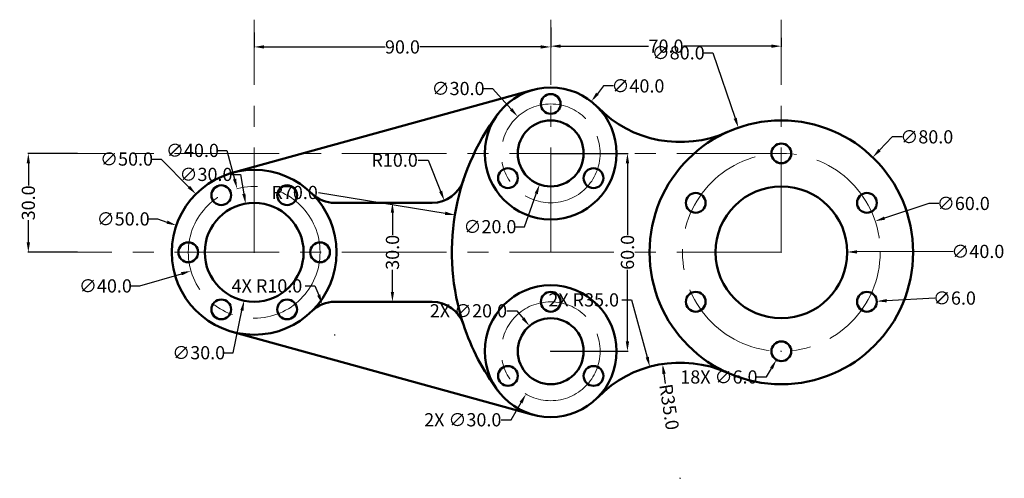
# Model space of a CAD drawing. Units: inches. Extents: x 1449 to 1748, y 643 to 782.
import ezdxf

# ---------------------------------------------------------------- set-up
doc = ezdxf.new("R2010")
doc.units = ezdxf.units.IN
doc.header["$MEASUREMENT"] = 0
doc.linetypes.add('CENTER', pattern=[50.8, 31.75, -6.35, 6.35, -6.35])
doc.layers.add('M-CNTR', color=32, linetype='CENTER', lineweight=18, true_color=0xcd6928)
doc.layers.add('M-DIMS', color=2, linetype='Continuous', lineweight=25)
doc.layers.add('M-OUTL', color=7, linetype='Continuous', lineweight=50)
doc.styles.get("Standard").update_dxf_attribs({"font": 'arial.ttf'})
doc.dimstyles.get("Standard").update_dxf_attribs({"dimtxt": 4, "dimasz": 3, "dimexe": 0.18, "dimexo": 0.0625, "dimgap": 0.09, "dimtad": 0, "dimtoh": 1, "dimdec": 1, "dimzin": 0, "dimdsep": 46, "dimtxsty": 'Standard', "dimcen": 0.09, "dimadec": 0, "dimazin": 0, "dimtfac": 1, "dimtdec": 1, "dimtofl": 0, "dimtmove": 0, "dimatfit": 3, "dimfxl": 1, "dimtolj": 1, "dimtzin": 0, "dimarcsym": 0})

# ---------------------------------------------------------------- blocks, each defined once
blk = doc.blocks.new('*D1')
at = {"layer": 'Defpoints', "color": 0, "transparency": 16777216}
for p in [(1519.9, 778.16), (1609.9, 779.72), (1609.9, 773.74)]:
    blk.add_point(p, dxfattribs=at)
at = {"layer": 'M-DIMS', "color": 0, "lineweight": -2, "transparency": 16777216}
for p, q in [((1519.9, 778.1), (1519.9, 773.56)), ((1609.9, 779.66), (1609.9, 773.56)), ((1522.9, 773.74), (1559.62, 773.74)), ((1606.9, 773.74), (1570.17, 773.74))]:
    blk.add_line(p, q, dxfattribs=at)
at = {"layer": 'M-DIMS', "color": 0, "transparency": 16777216}
for points in [[(1522.9, 774.24), (1522.9, 773.24), (1519.9, 773.74)], [(1606.9, 774.24), (1606.9, 773.24), (1609.9, 773.74)]]:
    blk.add_solid(points, dxfattribs=at)
at = {"layer": 'M-DIMS', "color": 0, "transparency": 16777216, "insert": (1564.9, 773.74), "char_height": 4, "attachment_point": 5}
blk.add_mtext('\\A1;90.0', dxfattribs=at)
blk = doc.blocks.new('*D2')
at = {"layer": 'Defpoints', "color": 0, "transparency": 16777216}
for p in [(1609.9, 776.61), (1679.9, 776.61), (1679.9, 773.98)]:
    blk.add_point(p, dxfattribs=at)
at = {"layer": 'M-DIMS', "color": 0, "lineweight": -2, "transparency": 16777216}
for p, q in [((1609.9, 776.55), (1609.9, 773.8)), ((1679.9, 776.55), (1679.9, 773.8)), ((1612.9, 773.98), (1639.63, 773.98)), ((1676.9, 773.98), (1650.16, 773.98))]:
    blk.add_line(p, q, dxfattribs=at)
at = {"layer": 'M-DIMS', "color": 0, "transparency": 16777216}
for points in [[(1612.9, 774.48), (1612.9, 773.48), (1609.9, 773.98)], [(1676.9, 774.48), (1676.9, 773.48), (1679.9, 773.98)]]:
    blk.add_solid(points, dxfattribs=at)
at = {"layer": 'M-DIMS', "color": 0, "transparency": 16777216, "insert": (1644.9, 773.98), "char_height": 4, "attachment_point": 5}
blk.add_mtext('\\A1;70.0', dxfattribs=at)
blk = doc.blocks.new('*D3')
at = {"layer": 'Defpoints', "color": 0, "transparency": 16777216}
for p in [(1609.9, 741.45), (1609.9, 681.45), (1633.19, 681.45)]:
    blk.add_point(p, dxfattribs=at)
at = {"layer": 'M-DIMS', "color": 0, "lineweight": -2, "transparency": 16777216}
for p, q in [((1609.96, 741.45), (1633.37, 741.45)), ((1633.19, 738.45), (1633.19, 716.74)), ((1633.19, 684.45), (1633.19, 706.16)), ((1609.96, 681.45), (1633.37, 681.45))]:
    blk.add_line(p, q, dxfattribs=at)
at = {"layer": 'M-DIMS', "color": 0, "transparency": 16777216}
for points in [[(1632.69, 738.45), (1633.69, 738.45), (1633.19, 741.45)], [(1632.69, 684.45), (1633.69, 684.45), (1633.19, 681.45)]]:
    blk.add_solid(points, dxfattribs=at)
at = {"layer": 'M-DIMS', "color": 0, "transparency": 16777216, "insert": (1633.19, 711.45), "char_height": 4, "attachment_point": 5, "rotation": 90}
blk.add_mtext('\\A1;60.0', dxfattribs=at)
blk = doc.blocks.new('*D4')
at = {"layer": 'Defpoints', "color": 0, "transparency": 16777216}
for p in [(1707.63, 740.27), (1652.16, 682.62)]:
    blk.add_point(p, dxfattribs=at)
at = {"layer": 'M-DIMS', "color": 0, "lineweight": -2, "transparency": 16777216}
for p, q in [((1713.59, 746.47), (1709.71, 742.44)), ((1716.59, 746.47), (1713.59, 746.47)), ((1679.81, 711.45), (1679.99, 711.45)), ((1679.9, 711.36), (1679.9, 711.54))]:
    blk.add_line(p, q, dxfattribs=at)
at = {"layer": 'M-DIMS', "color": 0, "transparency": 16777216}
blk.add_solid([(1709.35, 742.78), (1710.07, 742.09), (1707.63, 740.27)], dxfattribs=at)
at = {"layer": 'M-DIMS', "color": 0, "transparency": 16777216, "insert": (1724.05, 746.47), "char_height": 4, "attachment_point": 5}
blk.add_mtext('\\A1;∅80.0', dxfattribs=at)
blk = doc.blocks.new('*D5')
at = {"layer": 'Defpoints', "color": 0, "transparency": 16777216}
for p in [(1708.37, 720.88), (1651.42, 702.02)]:
    blk.add_point(p, dxfattribs=at)
at = {"layer": 'M-DIMS', "color": 0, "lineweight": -2, "transparency": 16777216}
for p, q in [((1724.69, 726.28), (1711.22, 721.82)), ((1727.69, 726.28), (1724.69, 726.28)), ((1679.81, 711.45), (1679.99, 711.45)), ((1679.9, 711.36), (1679.9, 711.54))]:
    blk.add_line(p, q, dxfattribs=at)
at = {"layer": 'M-DIMS', "color": 0, "transparency": 16777216}
blk.add_solid([(1711.07, 722.3), (1711.38, 721.35), (1708.37, 720.88)], dxfattribs=at)
at = {"layer": 'M-DIMS', "color": 0, "transparency": 16777216, "insert": (1735.14, 726.28), "char_height": 4, "attachment_point": 5}
blk.add_mtext('\\A1;∅60.0', dxfattribs=at)
blk = doc.blocks.new('*D6')
at = {"layer": 'Defpoints', "color": 0, "transparency": 16777216}
for p in [(1659.9, 711.34), (1699.9, 711.55)]:
    blk.add_point(p, dxfattribs=at)
at = {"layer": 'M-DIMS', "color": 0, "lineweight": -2, "transparency": 16777216}
for p, q in [((1679.81, 711.45), (1679.99, 711.45)), ((1679.9, 711.36), (1679.9, 711.54)), ((1732.09, 711.72), (1702.9, 711.57))]:
    blk.add_line(p, q, dxfattribs=at)
at = {"layer": 'M-DIMS', "color": 0, "transparency": 16777216}
blk.add_solid([(1702.89, 712.07), (1702.9, 711.07), (1699.9, 711.55)], dxfattribs=at)
at = {"layer": 'M-DIMS', "color": 0, "transparency": 16777216, "insert": (1739.55, 711.72), "char_height": 4, "attachment_point": 5}
blk.add_mtext('\\A1;∅40.0', dxfattribs=at)
blk = doc.blocks.new('*D7')
at = {"layer": 'Defpoints', "color": 0, "transparency": 16777216}
for p in [(1708.87, 696.61), (1702.88, 696.29)]:
    blk.add_point(p, dxfattribs=at)
at = {"layer": 'M-DIMS', "color": 0, "lineweight": -2, "transparency": 16777216}
for p, q in [((1705.79, 696.45), (1705.97, 696.45)), ((1705.88, 696.36), (1705.88, 696.54)), ((1726.54, 697.57), (1711.87, 696.77))]:
    blk.add_line(p, q, dxfattribs=at)
at = {"layer": 'M-DIMS', "color": 0, "transparency": 16777216}
blk.add_solid([(1711.84, 697.27), (1711.89, 696.27), (1708.87, 696.61)], dxfattribs=at)
at = {"layer": 'M-DIMS', "color": 0, "transparency": 16777216, "insert": (1732.44, 697.57), "char_height": 4, "attachment_point": 5}
blk.add_mtext('\\A1;∅6.0', dxfattribs=at)
blk = doc.blocks.new('*D8')
at = {"layer": 'Defpoints', "color": 0, "transparency": 16777216}
for p in [(1622.22, 757.2), (1597.57, 725.7)]:
    blk.add_point(p, dxfattribs=at)
at = {"layer": 'M-DIMS', "color": 0, "lineweight": -2, "transparency": 16777216}
for p, q in [((1625.92, 761.92), (1624.07, 759.56)), ((1628.92, 761.92), (1625.92, 761.92)), ((1609.81, 741.45), (1609.99, 741.45)), ((1609.9, 741.36), (1609.9, 741.54))]:
    blk.add_line(p, q, dxfattribs=at)
at = {"layer": 'M-DIMS', "color": 0, "transparency": 16777216}
blk.add_solid([(1623.68, 759.87), (1624.47, 759.25), (1622.22, 757.2)], dxfattribs=at)
at = {"layer": 'M-DIMS', "color": 0, "transparency": 16777216, "insert": (1636.38, 761.92), "char_height": 4, "attachment_point": 5}
blk.add_mtext('\\A1;∅40.0', dxfattribs=at)
blk = doc.blocks.new('*D9')
at = {"layer": 'Defpoints', "color": 0, "transparency": 16777216}
for p in [(1599.88, 752.62), (1619.91, 730.28)]:
    blk.add_point(p, dxfattribs=at)
at = {"layer": 'M-DIMS', "color": 0, "lineweight": -2, "transparency": 16777216}
for p, q in [((1589.25, 761.13), (1592.25, 761.13)), ((1592.25, 761.13), (1597.88, 754.85)), ((1609.81, 741.45), (1609.99, 741.45)), ((1609.9, 741.36), (1609.9, 741.54))]:
    blk.add_line(p, q, dxfattribs=at)
at = {"layer": 'M-DIMS', "color": 0, "transparency": 16777216}
blk.add_solid([(1598.25, 755.18), (1597.51, 754.52), (1599.88, 752.62)], dxfattribs=at)
at = {"layer": 'M-DIMS', "color": 0, "transparency": 16777216, "insert": (1581.79, 761.13), "char_height": 4, "attachment_point": 5}
blk.add_mtext('\\A1;∅30.0', dxfattribs=at)
blk = doc.blocks.new('*D10')
at = {"layer": 'Defpoints', "color": 0, "transparency": 16777216}
for p in [(1613.28, 750.86), (1606.52, 732.04)]:
    blk.add_point(p, dxfattribs=at)
at = {"layer": 'M-DIMS', "color": 0, "lineweight": -2, "transparency": 16777216}
for p, q in [((1609.81, 741.45), (1609.99, 741.45)), ((1609.9, 741.36), (1609.9, 741.54)), ((1601.92, 719.23), (1605.5, 729.21)), ((1598.92, 719.23), (1601.92, 719.23))]:
    blk.add_line(p, q, dxfattribs=at)
at = {"layer": 'M-DIMS', "color": 0, "transparency": 16777216}
blk.add_solid([(1605.03, 729.38), (1605.97, 729.04), (1606.52, 732.04)], dxfattribs=at)
at = {"layer": 'M-DIMS', "color": 0, "transparency": 16777216, "insert": (1591.46, 719.23), "char_height": 4, "attachment_point": 5}
blk.add_mtext('\\A1;∅20.0', dxfattribs=at)
blk = doc.blocks.new('*D11')
at = {"layer": 'Defpoints', "color": 0, "transparency": 16777216}
for p in [(1643.84, 677.59), (1649.23, 643)]:
    blk.add_point(p, dxfattribs=at)
at = {"layer": 'M-DIMS', "color": 0, "lineweight": -2, "transparency": 16777216}
blk.add_line((1644.77, 671.66), (1644.31, 674.62), dxfattribs=at)
at = {"layer": 'M-DIMS', "color": 0, "transparency": 16777216}
blk.add_solid([(1644.8, 674.7), (1643.81, 674.55), (1643.84, 677.59)], dxfattribs=at)
at = {"layer": 'M-DIMS', "color": 0, "transparency": 16777216, "insert": (1645.87, 664.55), "char_height": 4, "attachment_point": 5, "rotation": 278.8489}
blk.add_mtext('\\A1;R35.0', dxfattribs=at)
blk = doc.blocks.new('*D12')
at = {"layer": 'Defpoints', "color": 0, "transparency": 16777216}
for p in [(1496.27, 719.62), (1543.52, 703.28)]:
    blk.add_point(p, dxfattribs=at)
at = {"layer": 'M-DIMS', "color": 0, "lineweight": -2, "transparency": 16777216}
for p, q in [((1487.6, 721.58), (1490.6, 721.58)), ((1490.6, 721.58), (1493.43, 720.6)), ((1519.81, 711.45), (1519.99, 711.45)), ((1519.9, 711.36), (1519.9, 711.54))]:
    blk.add_line(p, q, dxfattribs=at)
at = {"layer": 'M-DIMS', "color": 0, "transparency": 16777216}
blk.add_solid([(1493.6, 721.07), (1493.27, 720.13), (1496.27, 719.62)], dxfattribs=at)
at = {"layer": 'M-DIMS', "color": 0, "transparency": 16777216, "insert": (1480.14, 721.58), "char_height": 4, "attachment_point": 5}
blk.add_mtext('\\A1;∅50.0', dxfattribs=at)
blk = doc.blocks.new('*D13')
at = {"layer": 'Defpoints', "color": 0, "transparency": 16777216}
for p in [(1539.09, 717.08), (1500.71, 705.81)]:
    blk.add_point(p, dxfattribs=at)
at = {"layer": 'M-DIMS', "color": 0, "lineweight": -2, "transparency": 16777216}
for p, q in [((1519.81, 711.45), (1519.99, 711.45)), ((1519.9, 711.36), (1519.9, 711.54)), ((1485.2, 701.26), (1497.83, 704.97)), ((1482.2, 701.26), (1485.2, 701.26))]:
    blk.add_line(p, q, dxfattribs=at)
at = {"layer": 'M-DIMS', "color": 0, "transparency": 16777216}
blk.add_solid([(1497.69, 705.45), (1497.97, 704.49), (1500.71, 705.81)], dxfattribs=at)
at = {"layer": 'M-DIMS', "color": 0, "transparency": 16777216, "insert": (1474.75, 701.26), "char_height": 4, "attachment_point": 5}
blk.add_mtext('\\A1;∅40.0', dxfattribs=at)
blk = doc.blocks.new('*D14')
at = {"layer": 'Defpoints', "color": 0, "transparency": 16777216}
for p in [(1522.97, 726.13), (1516.82, 696.77)]:
    blk.add_point(p, dxfattribs=at)
at = {"layer": 'M-DIMS', "color": 0, "lineweight": -2, "transparency": 16777216}
for p, q in [((1519.81, 711.45), (1519.99, 711.45)), ((1519.9, 711.36), (1519.9, 711.54)), ((1513.51, 681), (1516.2, 693.83)), ((1510.51, 681), (1513.51, 681))]:
    blk.add_line(p, q, dxfattribs=at)
at = {"layer": 'M-DIMS', "color": 0, "transparency": 16777216}
blk.add_solid([(1515.71, 693.93), (1516.69, 693.73), (1516.82, 696.77)], dxfattribs=at)
at = {"layer": 'M-DIMS', "color": 0, "transparency": 16777216, "insert": (1503.06, 681), "char_height": 4, "attachment_point": 5}
blk.add_mtext('\\A1;∅30.0', dxfattribs=at)
blk = doc.blocks.new('*D15')
at = {"layer": 'Defpoints', "color": 0, "transparency": 16777216}
for p in [(1561.86, 726.45), (1561.86, 696.45), (1561.86, 696.45)]:
    blk.add_point(p, dxfattribs=at)
at = {"layer": 'M-DIMS', "color": 0, "lineweight": -2, "transparency": 16777216}
for p, q in [((1561.92, 726.45), (1562.04, 726.45)), ((1561.86, 723.45), (1561.86, 716.73)), ((1561.86, 699.45), (1561.86, 706.17)), ((1561.92, 696.45), (1562.04, 696.45))]:
    blk.add_line(p, q, dxfattribs=at)
at = {"layer": 'M-DIMS', "color": 0, "transparency": 16777216}
for points in [[(1561.36, 723.45), (1562.36, 723.45), (1561.86, 726.45)], [(1561.36, 699.45), (1562.36, 699.45), (1561.86, 696.45)]]:
    blk.add_solid(points, dxfattribs=at)
at = {"layer": 'M-DIMS', "color": 0, "transparency": 16777216, "insert": (1561.86, 711.45), "char_height": 4, "attachment_point": 5, "rotation": 90}
blk.add_mtext('\\A1;30.0', dxfattribs=at)
blk = doc.blocks.new('*D16')
at = {"layer": 'Defpoints', "color": 0, "transparency": 16777216}
for p in [(1573.9, 736.45), (1577.61, 727.16)]:
    blk.add_point(p, dxfattribs=at)
at = {"layer": 'M-DIMS', "color": 0, "lineweight": -2, "transparency": 16777216}
for p, q in [((1569.72, 739.41), (1572.72, 739.41)), ((1572.72, 739.41), (1576.5, 729.95))]:
    blk.add_line(p, q, dxfattribs=at)
at = {"layer": 'M-DIMS', "color": 0, "transparency": 16777216}
blk.add_solid([(1576.96, 730.13), (1576.03, 729.76), (1577.61, 727.16)], dxfattribs=at)
at = {"layer": 'M-DIMS', "color": 0, "transparency": 16777216, "insert": (1562.53, 739.41), "char_height": 4, "attachment_point": 5}
blk.add_mtext('\\A1;R10.0', dxfattribs=at)
blk = doc.blocks.new('BOLT-HOLE-D6')
blk.add_circle((0, 0), 3)
blk = doc.blocks.new('MOUNTING-BOSS-3HOLE')
for centre, radius in [((0, 0), 20), ((0, 15), 3), ((0, 0), 10), ((-12.99, -7.5), 3), ((12.99, -7.5), 3)]:
    blk.add_circle(centre, radius)
blk = doc.blocks.new('*D19')
at = {"layer": 'Defpoints', "color": 0, "transparency": 16777216}
for p in [(1451.35, 741.45), (1466.35, 741.45), (1466.35, 711.45)]:
    blk.add_point(p, dxfattribs=at)
at = {"layer": 'M-DIMS', "color": 0, "lineweight": -2, "transparency": 16777216}
for p, q in [((1466.29, 741.45), (1451.17, 741.45)), ((1451.35, 738.45), (1451.35, 731.73)), ((1451.35, 714.45), (1451.35, 721.17)), ((1466.29, 711.45), (1451.17, 711.45))]:
    blk.add_line(p, q, dxfattribs=at)
at = {"layer": 'M-DIMS', "color": 0, "transparency": 16777216}
for points in [[(1450.85, 738.45), (1451.85, 738.45), (1451.35, 741.45)], [(1450.85, 714.45), (1451.85, 714.45), (1451.35, 711.45)]]:
    blk.add_solid(points, dxfattribs=at)
at = {"layer": 'M-DIMS', "color": 0, "transparency": 16777216, "insert": (1451.35, 726.45), "char_height": 4, "attachment_point": 5, "rotation": 90}
blk.add_mtext('\\A1;30.0', dxfattribs=at)
blk = doc.blocks.new('*D20')
at = {"layer": 'Defpoints', "color": 0, "transparency": 16777216}
for p in [(1580.82, 722.8), (1649.9, 711.45)]:
    blk.add_point(p, dxfattribs=at)
at = {"layer": 'M-DIMS', "color": 0, "lineweight": -2, "transparency": 16777216}
for p, q in [((1539.38, 729.61), (1577.86, 723.28)), ((1649.81, 711.45), (1649.99, 711.45)), ((1649.9, 711.36), (1649.9, 711.54))]:
    blk.add_line(p, q, dxfattribs=at)
at = {"layer": 'M-DIMS', "color": 0, "transparency": 16777216}
blk.add_solid([(1577.94, 723.78), (1577.78, 722.79), (1580.82, 722.8)], dxfattribs=at)
at = {"layer": 'M-DIMS', "color": 0, "transparency": 16777216, "insert": (1532.18, 729.61), "char_height": 4, "attachment_point": 5}
blk.add_mtext('\\A1;R70.0', dxfattribs=at)
blk = doc.blocks.new('*D21')
at = {"layer": 'Defpoints', "color": 0, "transparency": 16777216}
for p in [(1540.61, 695.71), (1544.39, 686.45)]:
    blk.add_point(p, dxfattribs=at)
at = {"layer": 'M-DIMS', "color": 0, "lineweight": -2, "transparency": 16777216}
for p, q in [((1535.34, 701.26), (1538.34, 701.26)), ((1538.34, 701.26), (1539.48, 698.48)), ((1544.3, 686.45), (1544.48, 686.45)), ((1544.39, 686.36), (1544.39, 686.54))]:
    blk.add_line(p, q, dxfattribs=at)
at = {"layer": 'M-DIMS', "color": 0, "transparency": 16777216}
blk.add_solid([(1539.94, 698.67), (1539.01, 698.3), (1540.61, 695.71)], dxfattribs=at)
at = {"layer": 'M-DIMS', "color": 0, "transparency": 16777216, "insert": (1523.77, 701.26), "char_height": 4, "attachment_point": 5}
blk.add_mtext('\\A1;4X R10.0', dxfattribs=at)
blk = doc.blocks.new('*D22')
at = {"layer": 'Defpoints', "color": 0, "transparency": 16777216}
for p in [(1639.98, 676.76), (1649.23, 643)]:
    blk.add_point(p, dxfattribs=at)
at = {"layer": 'M-DIMS', "color": 0, "lineweight": -2, "transparency": 16777216}
for p, q in [((1631.44, 697.02), (1634.44, 697.02)), ((1634.44, 697.02), (1639.19, 679.66)), ((1649.14, 643), (1649.32, 643)), ((1649.23, 642.91), (1649.23, 643.09))]:
    blk.add_line(p, q, dxfattribs=at)
at = {"layer": 'M-DIMS', "color": 0, "transparency": 16777216}
blk.add_solid([(1639.67, 679.79), (1638.71, 679.52), (1639.98, 676.76)], dxfattribs=at)
at = {"layer": 'M-DIMS', "color": 0, "transparency": 16777216, "insert": (1619.91, 697.02), "char_height": 4, "attachment_point": 5}
blk.add_mtext('\\A1;2X R35.0', dxfattribs=at)
blk = doc.blocks.new('*D23')
at = {"layer": 'Defpoints', "color": 0, "transparency": 16777216}
for p in [(1502.22, 729.13), (1537.57, 693.77)]:
    blk.add_point(p, dxfattribs=at)
at = {"layer": 'M-DIMS', "color": 0, "lineweight": -2, "transparency": 16777216}
for p, q in [((1488.62, 739.74), (1491.62, 739.74)), ((1491.62, 739.74), (1500.1, 731.25)), ((1519.81, 711.45), (1519.99, 711.45)), ((1519.9, 711.36), (1519.9, 711.54))]:
    blk.add_line(p, q, dxfattribs=at)
at = {"layer": 'M-DIMS', "color": 0, "transparency": 16777216}
blk.add_solid([(1500.45, 731.6), (1499.75, 730.9), (1502.22, 729.13)], dxfattribs=at)
at = {"layer": 'M-DIMS', "color": 0, "transparency": 16777216, "insert": (1481.16, 739.74), "char_height": 4, "attachment_point": 5}
blk.add_mtext('\\A1;∅50.0', dxfattribs=at)
blk = doc.blocks.new('*D24')
at = {"layer": 'Defpoints', "color": 0, "transparency": 16777216}
for p in [(1514.72, 730.77), (1525.07, 692.13)]:
    blk.add_point(p, dxfattribs=at)
at = {"layer": 'M-DIMS', "color": 0, "lineweight": -2, "transparency": 16777216}
for p, q in [((1508.62, 742.36), (1511.62, 742.36)), ((1511.62, 742.36), (1513.94, 733.67)), ((1519.81, 711.45), (1519.99, 711.45)), ((1519.9, 711.36), (1519.9, 711.54))]:
    blk.add_line(p, q, dxfattribs=at)
at = {"layer": 'M-DIMS', "color": 0, "transparency": 16777216}
blk.add_solid([(1514.43, 733.79), (1513.46, 733.54), (1514.72, 730.77)], dxfattribs=at)
at = {"layer": 'M-DIMS', "color": 0, "transparency": 16777216, "insert": (1501.16, 742.36), "char_height": 4, "attachment_point": 5}
blk.add_mtext('\\A1;∅40.0', dxfattribs=at)
blk = doc.blocks.new('*D25')
at = {"layer": 'Defpoints', "color": 0, "transparency": 16777216}
for p in [(1517.29, 726.22), (1522.5, 696.68)]:
    blk.add_point(p, dxfattribs=at)
at = {"layer": 'M-DIMS', "color": 0, "lineweight": -2, "transparency": 16777216}
for p, q in [((1512.73, 735.08), (1515.73, 735.08)), ((1515.73, 735.08), (1516.77, 729.17)), ((1519.81, 711.45), (1519.99, 711.45)), ((1519.9, 711.36), (1519.9, 711.54))]:
    blk.add_line(p, q, dxfattribs=at)
at = {"layer": 'M-DIMS', "color": 0, "transparency": 16777216}
blk.add_solid([(1517.26, 729.26), (1516.28, 729.09), (1517.29, 726.22)], dxfattribs=at)
at = {"layer": 'M-DIMS', "color": 0, "transparency": 16777216, "insert": (1505.27, 735.08), "char_height": 4, "attachment_point": 5}
blk.add_mtext('\\A1;∅30.0', dxfattribs=at)
blk = doc.blocks.new('*D26')
at = {"layer": 'Defpoints', "color": 0, "transparency": 16777216}
for p in [(1617.4, 694.44), (1602.39, 668.46)]:
    blk.add_point(p, dxfattribs=at)
at = {"layer": 'M-DIMS', "color": 0, "lineweight": -2, "transparency": 16777216}
for p, q in [((1609.81, 681.45), (1609.99, 681.45)), ((1609.9, 681.36), (1609.9, 681.54)), ((1597.89, 660.66), (1600.89, 665.86)), ((1594.89, 660.66), (1597.89, 660.66))]:
    blk.add_line(p, q, dxfattribs=at)
at = {"layer": 'M-DIMS', "color": 0, "transparency": 16777216}
blk.add_solid([(1600.46, 666.11), (1601.33, 665.61), (1602.39, 668.46)], dxfattribs=at)
at = {"layer": 'M-DIMS', "color": 0, "transparency": 16777216, "insert": (1583.21, 660.66), "char_height": 4, "attachment_point": 5}
blk.add_mtext('\\A1;2X ∅30.0', dxfattribs=at)
blk = doc.blocks.new('*D27')
at = {"layer": 'Defpoints', "color": 0, "transparency": 16777216}
for p in [(1603.47, 689.11), (1616.32, 673.79)]:
    blk.add_point(p, dxfattribs=at)
at = {"layer": 'M-DIMS', "color": 0, "lineweight": -2, "transparency": 16777216}
for p, q in [((1596.61, 693.71), (1599.61, 693.71)), ((1599.61, 693.71), (1601.54, 691.41)), ((1609.81, 681.45), (1609.99, 681.45)), ((1609.9, 681.36), (1609.9, 681.54))]:
    blk.add_line(p, q, dxfattribs=at)
at = {"layer": 'M-DIMS', "color": 0, "transparency": 16777216}
blk.add_solid([(1601.92, 691.73), (1601.16, 691.09), (1603.47, 689.11)], dxfattribs=at)
at = {"layer": 'M-DIMS', "color": 0, "transparency": 16777216, "insert": (1584.93, 693.71), "char_height": 4, "attachment_point": 5}
blk.add_mtext('\\A1;2X ∅20.0', dxfattribs=at)
blk = doc.blocks.new('*D28')
at = {"layer": 'Defpoints', "color": 0, "transparency": 16777216}
for p in [(1666.87, 749.27), (1692.92, 673.63)]:
    blk.add_point(p, dxfattribs=at)
at = {"layer": 'M-DIMS', "color": 0, "lineweight": -2, "transparency": 16777216}
for p, q in [((1656.06, 771.96), (1659.06, 771.96)), ((1659.06, 771.96), (1665.89, 752.11)), ((1679.81, 711.45), (1679.99, 711.45)), ((1679.9, 711.36), (1679.9, 711.54))]:
    blk.add_line(p, q, dxfattribs=at)
at = {"layer": 'M-DIMS', "color": 0, "transparency": 16777216}
blk.add_solid([(1666.37, 752.27), (1665.42, 751.94), (1666.87, 749.27)], dxfattribs=at)
at = {"layer": 'M-DIMS', "color": 0, "transparency": 16777216, "insert": (1648.6, 771.96), "char_height": 4, "attachment_point": 5}
blk.add_mtext('\\A1;∅80.0', dxfattribs=at)
blk = doc.blocks.new('*D29')
at = {"layer": 'Defpoints', "color": 0, "transparency": 16777216}
for p in [(1681.39, 684.05), (1678.4, 678.85)]:
    blk.add_point(p, dxfattribs=at)
at = {"layer": 'M-DIMS', "color": 0, "lineweight": -2, "transparency": 16777216}
for p, q in [((1679.81, 681.45), (1679.99, 681.45)), ((1679.9, 681.36), (1679.9, 681.54)), ((1675.41, 673.65), (1676.9, 676.25)), ((1672.41, 673.65), (1675.41, 673.65))]:
    blk.add_line(p, q, dxfattribs=at)
at = {"layer": 'M-DIMS', "color": 0, "transparency": 16777216}
blk.add_solid([(1676.47, 676.5), (1677.34, 676), (1678.4, 678.85)], dxfattribs=at)
at = {"layer": 'M-DIMS', "color": 0, "transparency": 16777216, "insert": (1660.95, 673.65), "char_height": 4, "attachment_point": 5}
blk.add_mtext('\\A1;18X ∅6.0', dxfattribs=at)

msp = doc.modelspace()

# ---------------------------------------------------------------- linework, layer by layer
at = {"layer": 'M-CNTR'}
for p, q in [((1519.9, 711.45), (1519.9, 782)), ((1609.9, 711.45), (1609.9, 782)), ((1679.9, 711.45), (1679.9, 782)), ((1679.9, 741.45), (1466.35, 741.45)), ((1679.9, 711.45), (1466.35, 711.45))]:
    msp.add_line(p, q, dxfattribs=at)
for centre, radius in [((1609.9, 741.45), 15), ((1679.9, 711.45), 30), ((1519.9, 711.45), 20), ((1609.9, 681.45), 15)]:
    msp.add_circle(centre, radius, dxfattribs=at)
at = {"layer": 'M-OUTL'}
for p, q in [((1513.25, 735.55), (1604.58, 760.73)), ((1573.9, 726.45), (1544.39, 726.45)), ((1573.9, 696.45), (1544.39, 696.45)), ((1604.58, 662.17), (1513.25, 687.35))]:
    msp.add_line(p, q, dxfattribs=at)
for centre, radius in [((1679.9, 711.45), 40), ((1519.9, 711.45), 25), ((1679.9, 711.45), 20), ((1519.9, 711.45), 15)]:
    msp.add_circle(centre, radius, dxfattribs=at)
for centre, radius, start, end in [((1649.9, 711.45), 70, 143.1301, 198.21), ((1649.23, 779.89), 35, 224.3449, 294.1353), ((1573.9, 736.45), 10, 270, 341.79), ((1544.39, 736.45), 10, 225.5847, 270), ((1544.39, 686.45), 10, 90, 134.4153), ((1573.9, 686.45), 10, 18.21, 90), ((1649.9, 711.45), 70, 198.21, 216.8699), ((1649.23, 643), 35, 65.8647, 135.6551)]:
    msp.add_arc(centre, radius, start, end, dxfattribs=at)

# ---------------------------------------------------------------- block references
for name, p in [('MOUNTING-BOSS-3HOLE', (1609.9, 741.45)), ('BOLT-HOLE-D6', (1679.9, 741.45)), ('BOLT-HOLE-D6', (1509.9, 728.77)), ('BOLT-HOLE-D6', (1529.9, 728.77)), ('BOLT-HOLE-D6', (1653.91, 726.45)), ('BOLT-HOLE-D6', (1705.88, 726.45)), ('BOLT-HOLE-D6', (1499.9, 711.45)), ('BOLT-HOLE-D6', (1539.9, 711.45)), ('BOLT-HOLE-D6', (1653.91, 696.45)), ('BOLT-HOLE-D6', (1705.88, 696.45)), ('BOLT-HOLE-D6', (1509.9, 694.13)), ('BOLT-HOLE-D6', (1529.9, 694.13)), ('BOLT-HOLE-D6', (1679.9, 681.45))]:
    msp.add_blockref(name, p, dxfattribs=at)
at = {"layer": 'M-OUTL', "rotation": 120.0000000000027}
msp.add_blockref('MOUNTING-BOSS-3HOLE', (1609.9, 681.45), dxfattribs=at)

# ---------------------------------------------------------------- dimensions: what is measured, and where the dimension line sits
at = {"layer": 'M-DIMS'}
for base, p1, p2, picture, middle in [((1609.9, 773.74), (1519.9, 778.16), (1609.9, 779.72), '*D1', (1564.9, 773.74)), ((1679.9, 773.98), (1609.9, 776.61), (1679.9, 776.61), '*D2', (1644.9, 773.98))]:
    dim = msp.add_linear_dim(base=base, p1=p1, p2=p2, dimstyle='Standard', override={"dimclrd": 0, "dimclre": 0, "dimclrt": 0}, dxfattribs=at)
    dim.commit()
    dim.dimension.update_dxf_attribs({"geometry": picture, "text_midpoint": middle})
for p1, p2, override, picture, middle in [((1692.92, 673.63), (1666.87, 749.27), {"dimdec": 1, "dimlfac": 1, "dimrnd": 0, "dimzin": 0, "dimdsep": 46, "dimlunit": 2}, '*D28', (1648.6, 771.96)), ((1619.91, 730.28), (1599.88, 752.62), {"dimclrd": 0, "dimclre": 0, "dimclrt": 0}, '*D9', (1581.79, 761.13)), ((1613.28, 750.86), (1606.52, 732.04), {"dimclrd": 0, "dimclre": 0, "dimclrt": 0}, '*D10', (1591.46, 719.23)), ((1652.16, 682.62), (1707.63, 740.27), {"dimclrd": 0, "dimclre": 0, "dimclrt": 0}, '*D4', (1724.05, 746.47)), ((1525.07, 692.13), (1514.72, 730.77), {"dimdec": 1, "dimlfac": 1, "dimrnd": 0, "dimzin": 0, "dimdsep": 46, "dimlunit": 2}, '*D24', (1501.16, 742.36)), ((1537.57, 693.77), (1502.22, 729.13), {"dimdec": 1, "dimlfac": 1, "dimrnd": 0, "dimzin": 0, "dimdsep": 46, "dimlunit": 2}, '*D23', (1481.16, 739.74)), ((1522.5, 696.68), (1517.29, 726.22), {"dimdec": 1, "dimlfac": 1, "dimrnd": 0, "dimzin": 0, "dimdsep": 46, "dimlunit": 2}, '*D25', (1505.27, 735.08)), ((1651.42, 702.02), (1708.37, 720.88), {"dimclrd": 0, "dimclre": 0, "dimclrt": 0}, '*D5', (1735.14, 726.28)), ((1522.97, 726.13), (1516.82, 696.77), {"dimclrd": 0, "dimclre": 0, "dimclrt": 0}, '*D14', (1503.06, 681)), ((1539.09, 717.08), (1500.71, 705.81), {"dimclrd": 0, "dimclre": 0, "dimclrt": 0}, '*D13', (1474.75, 701.26)), ((1659.9, 711.34), (1699.9, 711.55), {"dimclrd": 0, "dimclre": 0, "dimclrt": 0}, '*D6', (1732.09, 711.72)), ((1702.88, 696.29), (1708.87, 696.61), {"dimclrd": 0, "dimclre": 0, "dimclrt": 0}, '*D7', (1726.54, 697.57))]:
    dim = msp.add_diameter_dim_2p(p1=p1, p2=p2, dimstyle='Standard', override=override, dxfattribs=at)
    dim.commit()
    dim.dimension.update_dxf_attribs({"geometry": picture, "text_midpoint": middle, "dimtype": 163})
for p1, p2, picture, middle in [((1597.57, 725.7), (1622.22, 757.2), '*D8', (1636.38, 761.92)), ((1543.52, 703.28), (1496.27, 719.62), '*D12', (1480.14, 721.58))]:
    dim = msp.add_diameter_dim_2p(p1=p1, p2=p2, dimstyle='Standard', override={"dimclrd": 0, "dimclre": 0, "dimclrt": 0}, dxfattribs=at)
    dim.commit()
    dim.dimension.update_dxf_attribs({"geometry": picture, "text_midpoint": middle})
for base, p1, p2, override, picture, middle in [((1451.35, 741.45), (1466.35, 711.45), (1466.35, 741.45), {"dimdec": 1, "dimlfac": 1, "dimrnd": 0, "dimzin": 0, "dimdsep": 46, "dimlunit": 2}, '*D19', (1451.35, 726.45)), ((1633.19, 681.45), (1609.9, 741.45), (1609.9, 681.45), {"dimclrd": 0, "dimclre": 0, "dimclrt": 0}, '*D3', (1633.19, 711.45)), ((1561.86, 696.45), (1561.86, 726.45), (1561.86, 696.45), {"dimclrd": 0, "dimclre": 0, "dimclrt": 0}, '*D15', (1561.86, 711.45))]:
    dim = msp.add_linear_dim(base=base, p1=p1, p2=p2, angle=90, dimstyle='Standard', override=override, dxfattribs=at)
    dim.commit()
    dim.dimension.update_dxf_attribs({"geometry": picture, "text_midpoint": middle})
for center, mpoint, override, picture, middle in [((1573.9, 736.45), (1577.61, 727.16), {"dimclrd": 0, "dimclre": 0, "dimclrt": 0}, '*D16', (1562.53, 739.41)), ((1649.9, 711.45), (1580.82, 722.8), {"dimdec": 1, "dimlfac": 1, "dimrnd": 0, "dimzin": 0, "dimdsep": 46, "dimlunit": 2}, '*D20', (1539.38, 729.61)), ((1649.23, 643), (1643.84, 677.59), {"dimclrd": 0, "dimclre": 0, "dimclrt": 0}, '*D11', (1645.87, 664.55))]:
    dim = msp.add_radius_dim(center=center, mpoint=mpoint, dimstyle='Standard', override=override, dxfattribs=at)
    dim.commit()
    dim.dimension.update_dxf_attribs({"geometry": picture, "text_midpoint": middle, "dimtype": 164})
for center, mpoint, text, picture, middle in [((1544.39, 686.45), (1540.61, 695.71), '4X <>', '*D21', (1523.77, 701.26)), ((1649.23, 643), (1639.98, 676.76), '2X <>', '*D22', (1619.91, 697.02))]:
    dim = msp.add_radius_dim(center=center, mpoint=mpoint, text=text, dimstyle='Standard', override={"dimdec": 1, "dimlfac": 1, "dimrnd": 0, "dimzin": 0, "dimdsep": 46, "dimlunit": 2}, dxfattribs=at)
    dim.commit()
    dim.dimension.update_dxf_attribs({"geometry": picture, "text_midpoint": middle, "dimtype": 164})
for p1, p2, text, picture, middle in [((1616.32, 673.79), (1603.47, 689.11), '2X <>', '*D27', (1584.93, 693.71)), ((1681.39, 684.05), (1678.4, 678.85), '18X <>', '*D29', (1660.95, 673.65))]:
    dim = msp.add_diameter_dim_2p(p1=p1, p2=p2, text=text, dimstyle='Standard', override={"dimdec": 1, "dimlfac": 1, "dimrnd": 0, "dimzin": 0, "dimdsep": 46, "dimlunit": 2}, dxfattribs=at)
    dim.commit()
    dim.dimension.update_dxf_attribs({"geometry": picture, "text_midpoint": middle})
dim = msp.add_diameter_dim_2p(p1=(1617.4, 694.44), p2=(1602.39, 668.46), text='2X <>', dimstyle='Standard', override={"dimdec": 1, "dimlfac": 1, "dimrnd": 0, "dimzin": 0, "dimdsep": 46, "dimlunit": 2}, dxfattribs=at)
dim.commit()
dim.dimension.update_dxf_attribs({"geometry": '*D26', "text_midpoint": (1583.21, 660.66), "dimtype": 163})

doc.saveas('drawing.dxf')
